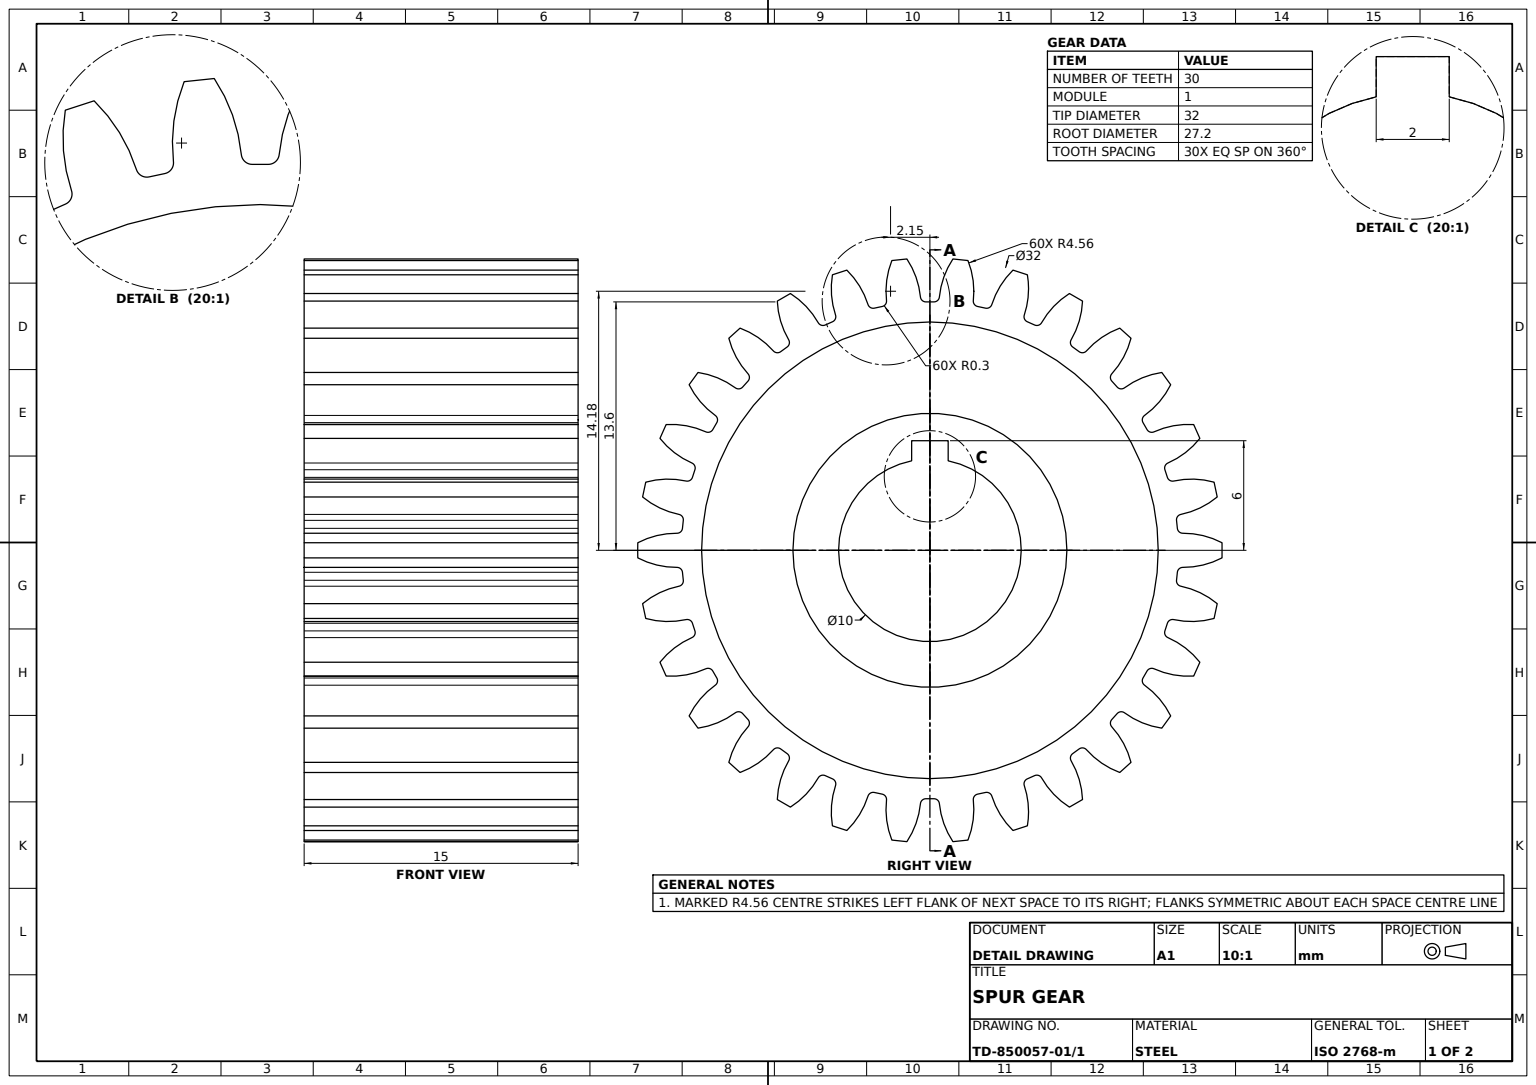
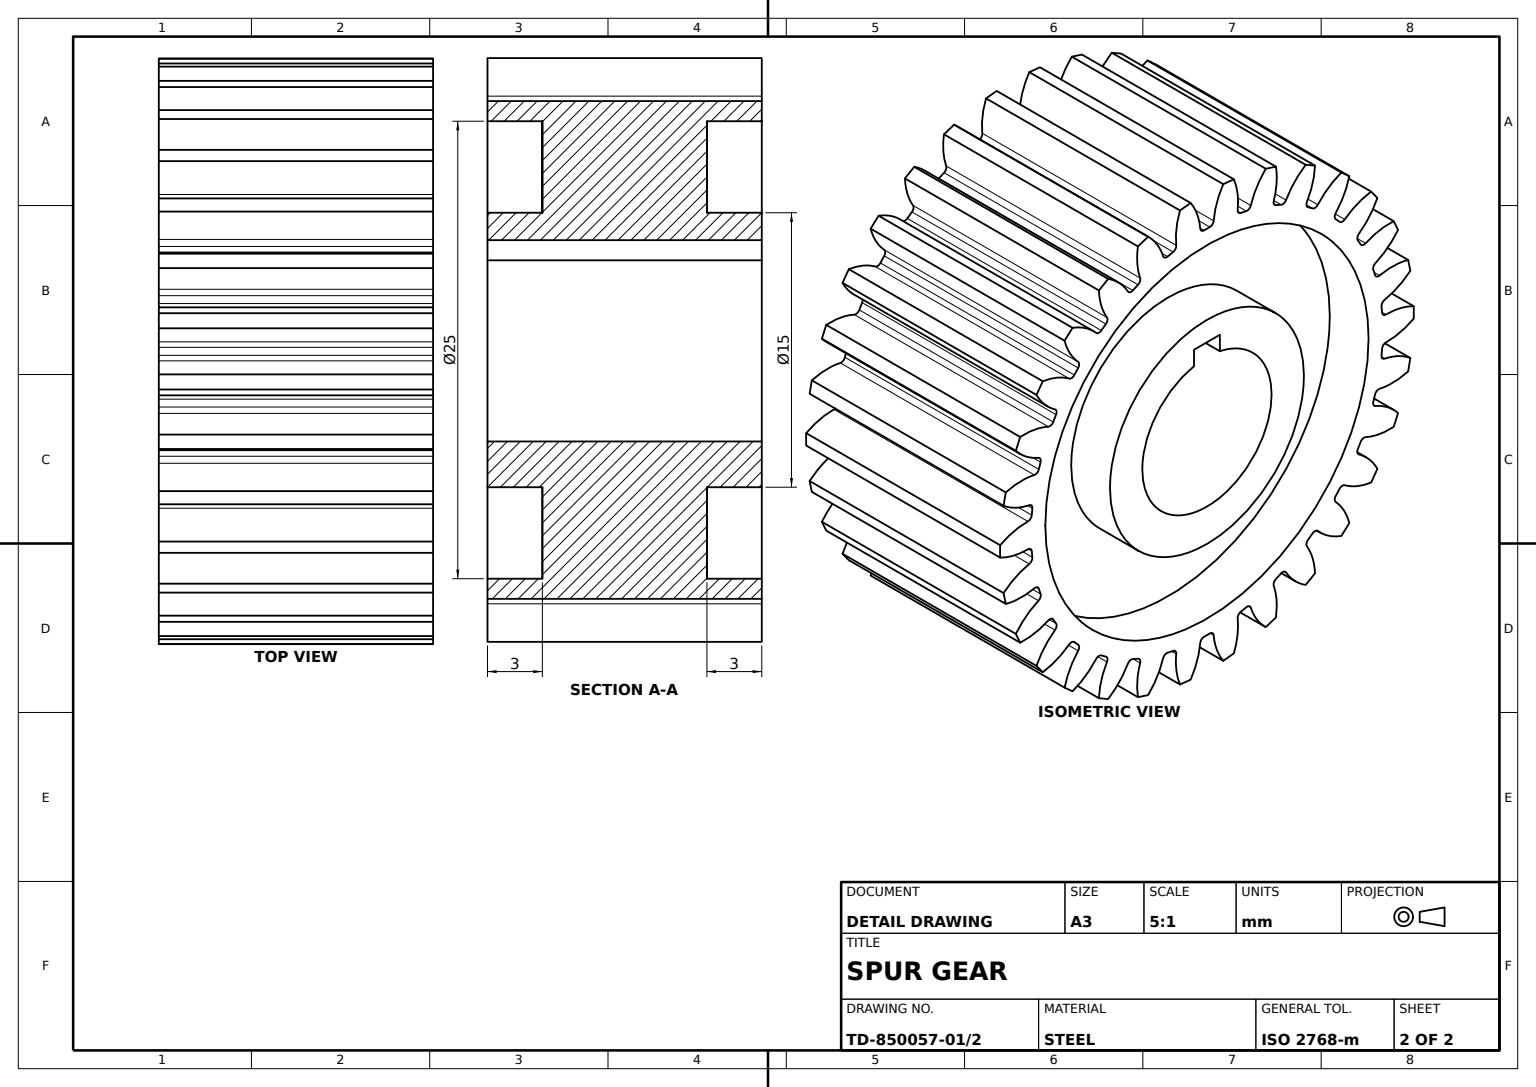
SolidWorks part; units mm, degrees
material "Plain Carbon Steel"
ref_plane "Front Plane" through (0, 0, 0) normal (0, 0, 1) x (1, 0, 0)
ref_plane "Top Plane" through (0, 0, 0) normal (0, 1, 0) x (1, 0, 0)
ref_plane "Right Plane" through (0, 0, 0) normal (1, 0, 0) x (0, 0, -1)
sketch "Gear Blank Sketch" plane through (0, 0, 0) normal (1, 0, 0) x (0, 0, -1)
  circle A0 centre (0, 0) radius 16
  dimension "D1" = 32
extrude "Gear Blank Ø32x15" add sketch "Gear Blank Sketch" along normal mid plane 15
sketch "Keyed Bore Sketch" plane through (7.5, 0, 0) normal (1, 0, 0) x (0, 0, -1)
  line L1 (-1, 6) -> (1, 6)
  line L2 (-1, 6) -> (-1, 4.899)
  line L4 (1, 6) -> (1, 4.899)
  line L5 (-1, 6) -> (0, 5) construction
  line L6 (0, 5) -> (1, 6) construction
  arc A0 (-1, 4.899) -> (1, 4.899) centre (0, 0) ccw
  point P3 (0, 5)
  dimension "D1" = 10
  dimension "D2" = 2
extrude "Keyed Bore Ø10" cut sketch "Keyed Bore Sketch" against normal through all
sketch "Hub Recess Sketch" plane through (7.5, 0, 0) normal (1, 0, 0) x (0, 0, -1)
  circle A0 centre (0, 0) radius 7.5
  circle A1 centre (0, 0) radius 12.5
  dimension "D1" = 25
  dimension "D2" = 15
extrude "Hub Recess Ø25-Ø15 x3" cut sketch "Hub Recess Sketch" against normal blind 3
mirror "Hub Recess Mirror" about plane through (0, 0, 0) normal (1, 0, 0) of "Hub Recess Ø25-Ø15 x3"
sketch "Tooth Space Sketch" plane through (7.5, 0, 0) normal (1, 0, 0) x (0, 0, -1)
  line L0 (0, 0) -> (0, 27.2) construction
  line L1 (-0.2199, 13.6) -> (0.2199, 13.6)
  arc A0 (0.5184, 13.8707) -> (2.08, 16.88) centre (5.0567, 13.4256) cw
  arc A1 (-0.5184, 13.8707) -> (-2.08, 16.88) centre (-5.0567, 13.4256) ccw
  arc A2 (-2.08, 16.88) -> (2.08, 16.88) centre (0, -0.9994) cw
  arc A3 (0.2199, 13.6) -> (0.5184, 13.8707) centre (0.2199, 13.9) ccw
  arc A4 (-0.5184, 13.8707) -> (-0.2199, 13.6) centre (-0.2199, 13.9) ccw
  point P10 (0, 13.6)
  point P13 (0.5, 13.6)
  point P16 (-0.5, 13.6)
  dimension "D5" = 4.56
  dimension "D6" = 18
  dimension "D7" = 0.3
  dimension "D1" = 0.5
  dimension "D2" = 13.6
  dimension "D3" = 1.58
  dimension "D4" = 3.28
extrude "Tooth Space Cut" cut sketch "Tooth Space Sketch" against normal through all and the other way through all
pattern_circular "Tooth Pattern 30x" count 30 over 360 about axis through (0, 0, 0) along (1, 0, 0) of "Tooth Space Cut"
